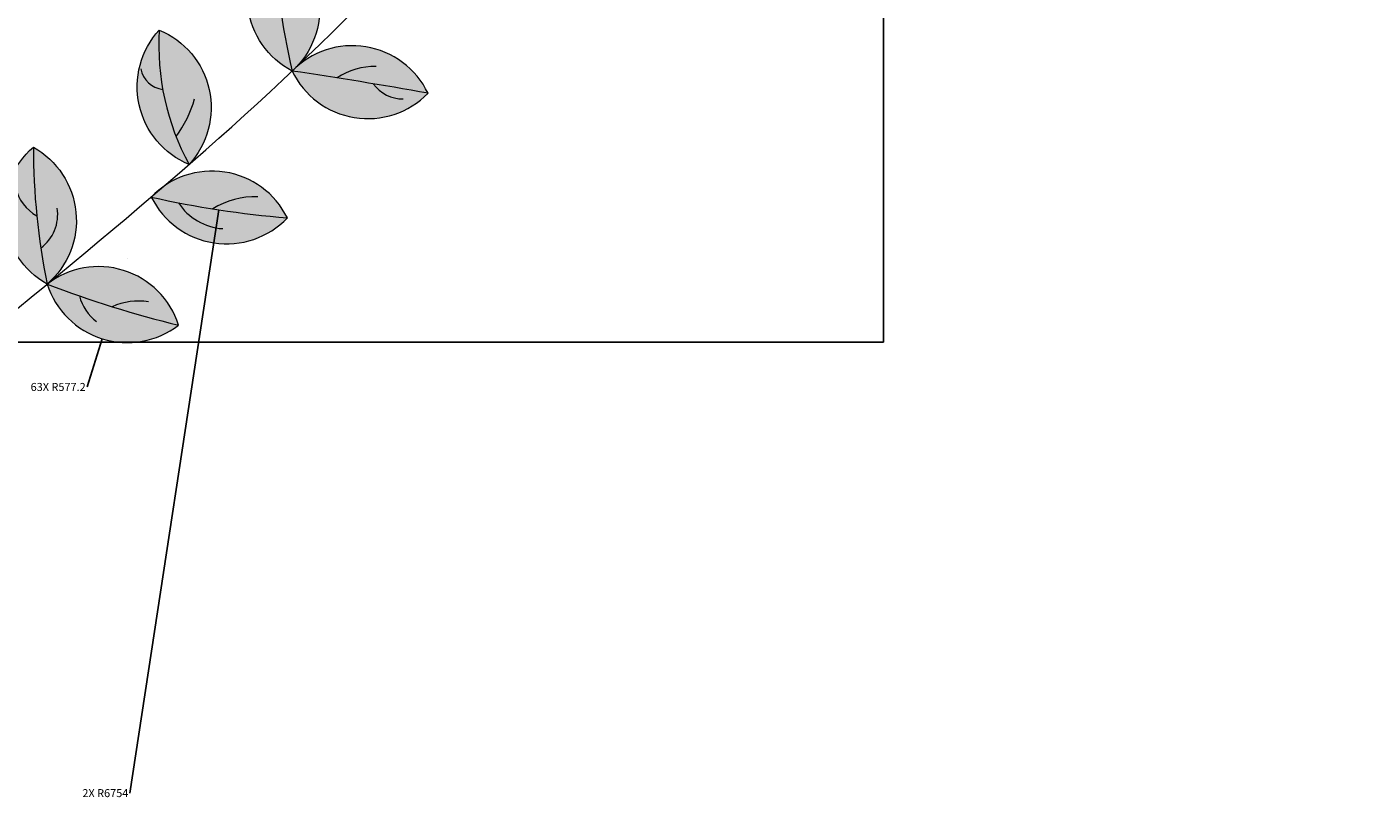
# Model space of a CAD drawing. Units: millimetres. Extents: x 8570 to 49085, y 3782 to 24863.
# Tile 13 of 15: x 39837 to 49085, y 4304 to 9648. Entities that reach past the tile are written whole.
import ezdxf

# ---------------------------------------------------------------- set-up
doc = ezdxf.new("R2010")
doc.units = ezdxf.units.MM
doc.header["$MEASUREMENT"] = 0
doc.header["$PDMODE"] = 3
for name, color, linetype, lineweight in [('A-ANNO-DIMS', 2, 'Continuous', 18), ('A-DETL-FOLI', 7, 'Continuous', 13), ('A-DETL-PATT', 3, 'Continuous', 13), ('A-DETL-STEM', 28, 'Continuous', 18)]:
    doc.layers.add(name, color=color, linetype=linetype, lineweight=lineweight)
doc.styles.get("Standard").update_dxf_attribs({"font": 'arial.ttf'})
doc.dimstyles.get("Standard").update_dxf_attribs({"dimtxt": 55, "dimasz": 0.18, "dimexe": 0.18, "dimexo": 0.0625, "dimgap": 0.09, "dimtad": 0, "dimtih": 1, "dimtoh": 1, "dimdec": 0, "dimzin": 0, "dimdsep": 46, "dimtxsty": 'Standard', "dimcen": 0.09, "dimadec": 0, "dimazin": 0, "dimtfac": 1, "dimtdec": 0, "dimtofl": 0, "dimtmove": 0, "dimatfit": 3, "dimfxl": 1, "dimtolj": 1, "dimtzin": 0, "dimarcsym": 0})

# ---------------------------------------------------------------- blocks, each defined once
blk = doc.blocks.new('*D76')
at = {"layer": 'A-ANNO-DIMS', "color": 0, "lineweight": -2, "transparency": 16777216}
for p, q in [((45255.3, 15109.5), (45721.9, 15109.5)), ((45721.7, 15109.3), (45721.7, 11324.7)), ((45721.7, 7483.7), (45721.7, 11268.3)), ((39491.1, 7483.5), (45721.9, 7483.5))]:
    blk.add_line(p, q, dxfattribs=at)
at = {"layer": 'A-ANNO-DIMS', "color": 0, "transparency": 16777216}
for points in [[(45721.6, 15109.3), (45721.7, 15109.3), (45721.7, 15109.5)], [(45721.6, 7483.7), (45721.7, 7483.7), (45721.7, 7483.5)]]:
    blk.add_solid(points, dxfattribs=at)
at = {"layer": 'Defpoints', "color": 0, "transparency": 16777216}
for p in [(45255.2, 15109.5), (45721.7, 15109.5), (39491, 7483.5)]:
    blk.add_point(p, dxfattribs=at)
at = {"layer": 'A-ANNO-DIMS', "color": 0, "transparency": 16777216, "insert": (45721.7, 11296.5), "char_height": 55, "attachment_point": 5}
blk.add_mtext('\\A1;7626', dxfattribs=at)
blk = doc.blocks.new('*D95')
at = {"layer": 'A-ANNO-DIMS', "color": 0, "lineweight": -2, "transparency": 16777216}
for p, q in [((48826.8, 12322.2), (42401, 10673.8)), ((31690.9, 7926.2), (31691.1, 7926.2)), ((31691, 7926.2), (31691, 7926.3))]:
    blk.add_line(p, q, dxfattribs=at)
at = {"layer": 'A-ANNO-DIMS', "color": 0, "transparency": 16777216}
blk.add_solid([(42401, 10673.8), (42401, 10673.7), (42400.9, 10673.7)], dxfattribs=at)
at = {"layer": 'Defpoints', "color": 0, "transparency": 16777216}
for p in [(42400.9, 10673.7), (31691, 7926.2)]:
    blk.add_point(p, dxfattribs=at)
at = {"layer": 'A-ANNO-DIMS', "color": 0, "transparency": 16777216, "insert": (48956.7, 12322.2), "char_height": 55, "attachment_point": 5}
blk.add_mtext('\\A1;R11057', dxfattribs=at)
blk = doc.blocks.new('*D96')
at = {"layer": 'A-ANNO-DIMS', "color": 0, "lineweight": -2, "transparency": 16777216}
for p, q in [((42176.7, 15068.1), (42176.9, 15068.1)), ((42176.8, 15068), (42176.8, 15068.2)), ((40544.1, 4385.9), (41156.3, 8391.6)), ((40543.9, 4385.9), (40544.1, 4385.9))]:
    blk.add_line(p, q, dxfattribs=at)
at = {"layer": 'A-ANNO-DIMS', "color": 0, "transparency": 16777216}
blk.add_solid([(41156.3, 8391.6), (41156.3, 8391.6), (41156.3, 8391.7)], dxfattribs=at)
at = {"layer": 'Defpoints', "color": 0, "transparency": 16777216}
for p in [(42176.8, 15068.1), (41156.3, 8391.7)]:
    blk.add_point(p, dxfattribs=at)
at = {"layer": 'A-ANNO-DIMS', "color": 0, "transparency": 16777216, "insert": (40375.9, 4385.9), "char_height": 55, "attachment_point": 5}
blk.add_mtext('\\A1;2X R6754', dxfattribs=at)
blk = doc.blocks.new('*D101')
at = {"layer": 'A-ANNO-DIMS', "color": 0, "lineweight": -2, "transparency": 16777216}
for p, q in [((40526.5, 8056.9), (40526.6, 8056.9)), ((40526.5, 8056.8), (40526.5, 8056.9)), ((40251.4, 7175.3), (40354.6, 7505.7)), ((40251.3, 7175.3), (40251.4, 7175.3))]:
    blk.add_line(p, q, dxfattribs=at)
at = {"layer": 'A-ANNO-DIMS', "color": 0, "transparency": 16777216}
blk.add_solid([(40354.5, 7505.7), (40354.6, 7505.7), (40354.6, 7505.9)], dxfattribs=at)
at = {"layer": 'Defpoints', "color": 0, "transparency": 16777216}
for p in [(40526.5, 8056.9), (40354.6, 7505.9)]:
    blk.add_point(p, dxfattribs=at)
at = {"layer": 'A-ANNO-DIMS', "color": 0, "transparency": 16777216, "insert": (40051.7, 7175.3), "char_height": 55, "attachment_point": 5}
blk.add_mtext('\\A1;63X R577.2', dxfattribs=at)

msp = doc.modelspace()

# ---------------------------------------------------------------- hatches: boundary and pattern name
at = {"layer": 'A-DETL-PATT'}
h = msp.add_hatch(color=256, dxfattribs=at)
h.dxf.hatch_style = 1
h.paths.add_polyline_path([(41539.85, 10282.96, 0.0525775), (41659.15, 9344.88, -0.0152167), (41684.42, 9369.28, 0.5013788)])
h = msp.add_hatch(color=256, dxfattribs=at)
h.dxf.hatch_style = 1
h.paths.add_polyline_path([(41423.54, 10136.32, 0.4210746), (41659.15, 9344.88, -0.0354074), (41557.06, 9974.44, -0.1348282)])
h = msp.add_hatch(color=256, dxfattribs=at)
h.dxf.hatch_style = 1
h.paths.add_polyline_path([(40746.58, 9626.63, 0.5205671), (40951, 8703.36, -0.1409243)])
h = msp.add_hatch(color=256, dxfattribs=at)
h.dxf.hatch_style = 1
h.paths.add_polyline_path([(40746.58, 9626.63, 0.1409243), (40951, 8703.36, 0.5205671)])
h = msp.add_hatch(color=256, dxfattribs=at)
h.dxf.hatch_style = 1
h.paths.add_polyline_path([(41684.42, 9369.28, -0.0152167), (41659.15, 9344.88, -0.0070162), (42592.46, 9192.63, 0.5013788)])
h = msp.add_hatch(color=256, dxfattribs=at)
h.dxf.hatch_style = 1
h.paths.add_polyline_path([(41659.15, 9344.88, 0.5205671), (42592.46, 9192.63, 0.0070162)])
h = msp.add_hatch(color=256, dxfattribs=at)
h.dxf.hatch_style = 1
h.paths.add_polyline_path([(39881.17, 8822.47, 0.5205671), (39976.57, 7881.66, -0.0505737)])
h = msp.add_hatch(color=256, dxfattribs=at)
h.dxf.hatch_style = 1
h.paths.add_polyline_path([(39881.17, 8822.47, 0.0505737), (39976.57, 7881.66, 0.520567)])
h = msp.add_hatch(color=256, dxfattribs=at)
h.dxf.hatch_style = 1
edge = h.paths.add_edge_path()
edge.add_spline(control_points=[(40779.07, 8554.58), (40749.92, 8529.54), (40720.72, 8504.53), (40691.45, 8479.55)], knot_values=[1468.6434181, 1468.6434181, 1468.6434181, 1468.6434181, 1577.9808208, 1577.9808208, 1577.9808208, 1577.9808208], degree=3, periodic=0)
edge.add_arc((42176.8, 15068.1), 6753.9, 257.295444, 265.324191)
edge.add_arc((41108.82, 8080.85), 577.2, 26.309818, 124.840841)
h = msp.add_hatch(color=256, dxfattribs=at)
h.dxf.hatch_style = 1
h.paths.add_polyline_path([(40691.45, 8479.55, 0.5205671), (41626.23, 8336.68, -0.0350464)])
h = msp.add_hatch(color=256, dxfattribs=at)
h.dxf.hatch_style = 1
h.paths.add_polyline_path([(39976.57, 7881.66, 0.0328597), (40879.28, 7599.98, 0.5205671)])
h = msp.add_hatch(color=256, dxfattribs=at)
h.dxf.hatch_style = 1
h.paths.add_polyline_path([(39976.57, 7881.66, 0.520567), (40879.28, 7599.98, -0.0328597)])

# ---------------------------------------------------------------- linework, layer by layer
at = {"layer": 'A-DETL-FOLI'}
for points in [[(41659.15, 9344.88, -0.5205671), (41539.85, 10282.96, -0.5205671)], [(40951, 8703.36, -0.5205671), (40746.58, 9626.63, -0.5205671)], [(41659.15, 9344.88, 0.5205671), (42592.46, 9192.63, 0.5205671)], [(39976.57, 7881.66, -0.5205671), (39881.17, 8822.47, -0.5205671)], [(40691.45, 8479.55, 0.5205671), (41626.23, 8336.68, 0.5205671)], [(39976.57, 7881.66, 0.5205671), (40879.28, 7599.98, 0.5205671)]]:
    msp.add_lwpolyline(points, format="xyb", close=True, dxfattribs=at)
for centre, radius, start, end in [((46047.63, 10379.64), 4508.82, 181.228633, 193.267432), ((42454.15, 9520.44), 1710.88, 176.44123, 208.52741), ((40788.18, 9388.66), 170.45, 189.441328, 263.88078), ((36701.25, -23985.01), 33696.62, 79.931196, 81.539154), ((42225.34, 8913.92), 462.08, 88.661125, 123.884115), ((42418.9, 9402.71), 249.31, 215.70646, 270.831731), ((40257.58, 9354.52), 758.17, 322.780807, 344.606902), ((44567.67, 8822.47), 4686.5, 180, 191.580779), ((40061.17, 8620.56), 312.66, 193.8989, 240.051258), ((42176.8, 15068.1), 6753.9, 257.295444, 265.324191), ((41205.8, 8651.94), 390.09, 212.870315, 266.488336), ((41401.62, 7943.01), 538.45, 87.789477, 122.264346), ((39760.84, 8359.95), 287.73, 306.683544, 8.744496), ((42568.69, 14601.31), 7202.28, 248.905805, 256.433978), ((40512.65, 7884.53), 326.41, 194.889105, 232.969394), ((40601.16, 7344.06), 421.31, 80.265821, 114.971162)]:
    msp.add_arc(centre, radius, start, end, dxfattribs=at)
at = {"layer": 'A-DETL-STEM'}
msp.add_open_spline([(39491, 7483.5), (41497.86, 9125.36), (43912.02, 11100.44), (44441.22, 14010.96), (44530.5, 14502)], degree=3, knots=[0, 0, 0, 0, 7301.1442939, 8782.9420196, 8782.9420196, 8782.9420196, 8782.9420196], dxfattribs=at)

# ---------------------------------------------------------------- dimensions: what is measured, and where the dimension line sits
at = {"layer": 'A-ANNO-DIMS'}
dim = msp.add_linear_dim(base=(45721.68, 15109.49), p1=(39491, 7483.5), p2=(45255.2, 15109.49), angle=90, dimstyle='Standard', override={"dimdec": 0, "dimlfac": 1, "dimrnd": 0, "dimzin": 0, "dimdsep": 46, "dimlunit": 2}, dxfattribs=at)
dim.commit()
dim.dimension.update_dxf_attribs({"geometry": '*D76', "text_midpoint": (45721.68, 11296.49)})
for center, mpoint, text, override, picture, middle in [((42176.8, 15068.1), (41156.34, 8391.74), '2X <>', {"dimdec": 0, "dimlfac": 1, "dimrnd": 0, "dimzin": 0, "dimdsep": 46, "dimlunit": 2}, '*D96', (40375.91, 4385.92)), ((40526.54, 8056.86), (40354.61, 7505.86), '63X <>', {"dimdec": 1, "dimlfac": 1, "dimrnd": 0, "dimzin": 0, "dimdsep": 46, "dimlunit": 2}, '*D101', (40051.74, 7175.26))]:
    dim = msp.add_radius_dim(center=center, mpoint=mpoint, text=text, dimstyle='Standard', override=override, dxfattribs=at)
    dim.commit()
    dim.dimension.update_dxf_attribs({"geometry": picture, "text_midpoint": middle, "dimtype": 164})
dim = msp.add_radius_dim(center=(31690.99, 7926.25), mpoint=(42400.86, 10673.71), dimstyle='Standard', override={"dimdec": 0, "dimlfac": 1, "dimrnd": 0, "dimzin": 0, "dimdsep": 46, "dimlunit": 2}, dxfattribs=at)
dim.commit()
dim.dimension.update_dxf_attribs({"geometry": '*D95', "text_midpoint": (48826.79, 12322.19), "dimtype": 164})

doc.saveas('drawing.dxf')
